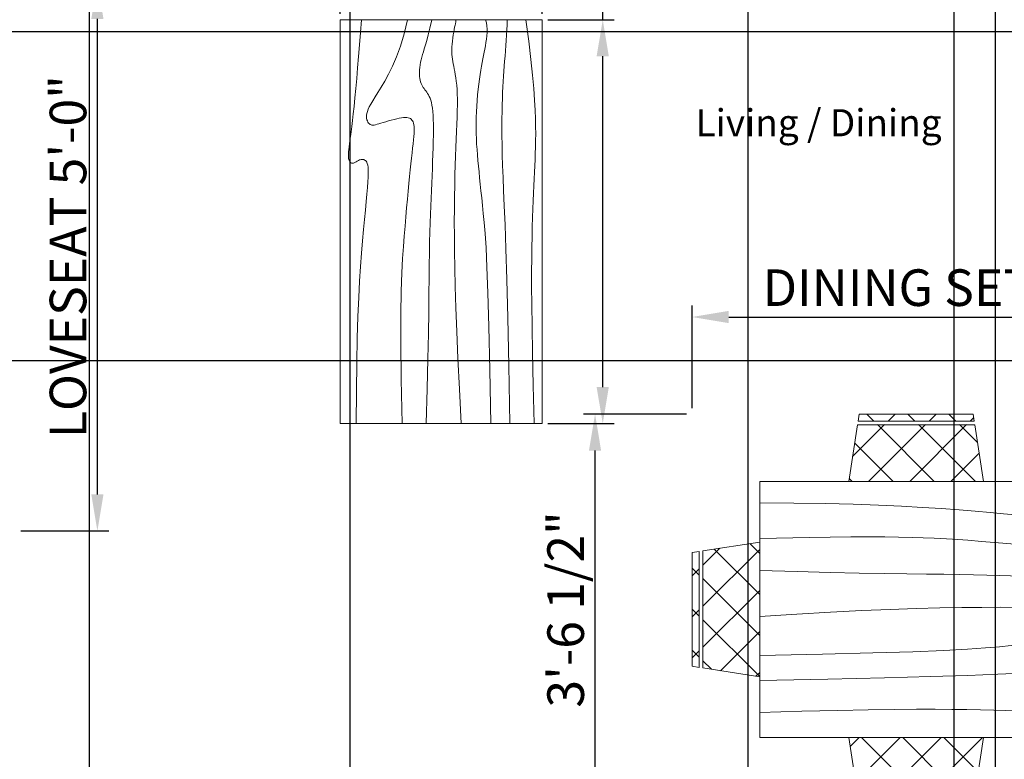
# Model space of a CAD drawing. Units: inches. Extents: x 1872 to 2380, y 714 to 1327.
# Tile 5 of 9: x 1994 to 2101, y 974 to 1055. Entities that reach past the tile are written whole.
import ezdxf

# ---------------------------------------------------------------- set-up
doc = ezdxf.new("R2010")
doc.units = ezdxf.units.IN
for name, color, linetype, lineweight in [('A-ANNO-DIMS', 2, 'Continuous', 18), ('A-AREA-IDEN', 7, 'Continuous', 18), ('A-FURN', 8, 'Continuous', 18)]:
    doc.layers.add(name, color=color, linetype=linetype, lineweight=lineweight)
doc.layers.add('A-FURN-PATT', color=254, linetype='Continuous', lineweight=13, true_color=0xf8ceb3)
doc.styles.get("Standard").update_dxf_attribs({"font": 'arial.ttf'})
doc.dimstyles.new('ISO-25', dxfattribs={"dimtxt": 4, "dimasz": 4, "dimexe": 1.25, "dimexo": 0.625, "dimtad": 1, "dimdec": 0, "dimlunit": 3, "dimtxsty": 'Standard', "dimcen": 2.5, "dimadec": 0, "dimazin": 0, "dimtfac": 1, "dimtdec": 0, "dimtmove": 0, "dimatfit": 3, "dimfxl": 1, "dimarcsym": 0})

# ---------------------------------------------------------------- blocks, each defined once
blk = doc.blocks.new('Table - Rectangular Woodgrain 60 x 30 in.')
for p, q in [((0, 0), (0, -30)), ((60, 0), (0, 0)), ((60, -30), (60, 0)), ((0, -30), (60, -30))]:
    blk.add_line(p, q)
for points in [[(0, -2.4), (4.8155, -2.418), (9.0302, -2.4688), (12.709, -2.5477), (15.9167, -2.65), (18.7181, -2.7711), (21.1781, -2.9063), (23.3616, -3.0508), (25.3333, -3.2), (27.1477, -3.3495), (28.8172, -3.4958), (30.3437, -3.636), (31.7291, -3.7667), (32.9756, -3.8849), (34.0849, -3.9875), (35.059, -4.0714), (35.9, -4.1334), (36.6114, -4.1711), (37.2041, -4.1854), (37.6906, -4.1779), (38.0833, -4.15), (38.3948, -4.1034), (38.6375, -4.0396), (38.8239, -3.9602), (38.9666, -3.8667), (39.0764, -3.7608), (39.1573, -3.6448), (39.2116, -3.521), (39.2416, -3.3917), (39.2498, -3.2593), (39.2385, -3.1261), (39.21, -2.9944), (39.1666, -2.8667), (39.111, -2.7447), (39.0468, -2.6281), (38.978, -2.5163), (38.9083, -2.4083), (38.8418, -2.3035), (38.7823, -2.201), (38.7337, -2.1001), (38.7, -2), (38.6844, -1.9003), (38.6875, -1.8021), (38.7094, -1.707), (38.75, -1.6167), (38.8094, -1.5326), (38.8875, -1.4563), (38.9844, -1.3893), (39.1, -1.3333), (39.2351, -1.2896), (39.3937, -1.2583), (39.5804, -1.2396), (39.8, -1.2333), (40.057, -1.2396), (40.3562, -1.2583), (40.7023, -1.2896), (41.1, -1.3333), (41.5547, -1.3895), (42.0755, -1.4573), (42.6721, -1.5361), (43.3542, -1.625), (44.1316, -1.7233), (45.014, -1.8302), (46.0114, -1.9449), (47.1333, -2.0667), (48.3862, -2.1947), (49.7625, -2.3281), (51.2513, -2.4663), (52.8416, -2.6083), (54.5226, -2.7535), (56.2833, -2.9011), (58.1127, -3.0501), (60, -3.2)], [(0, -9.2), (6.5759, -9.0858), (11.9385, -9.0365), (16.2527, -9.0418), (19.6833, -9.0917), (22.3952, -9.1759), (24.5531, -9.2844), (26.322, -9.4069), (27.8666, -9.5333), (29.3241, -9.6553), (30.7203, -9.7719), (32.0532, -9.8837), (33.3208, -9.9917), (34.5213, -10.0965), (35.6526, -10.199), (36.7128, -10.2999), (37.7, -10.4), (38.6129, -10.4996), (39.4531, -10.5969), (40.223, -10.6895), (40.925, -10.775), (41.5613, -10.8512), (42.1344, -10.9156), (42.6465, -10.966), (43.1, -11), (43.4976, -11.0158), (43.8437, -11.0136), (44.143, -10.9942), (44.4, -10.9583), (44.6195, -10.9069), (44.8062, -10.8406), (44.9648, -10.7603), (45.1, -10.6667), (45.2155, -10.5598), (45.3114, -10.4365), (45.3871, -10.2929), (45.4416, -10.125), (45.4743, -9.929), (45.4844, -9.7011), (45.4709, -9.4371), (45.4333, -9.1333), (45.3716, -8.7883), (45.2896, -8.4104), (45.1919, -8.0107), (45.0833, -7.6), (44.9685, -7.1893), (44.8521, -6.7896), (44.7388, -6.4117), (44.6333, -6.0667), (44.54, -5.7628), (44.4614, -5.4979), (44.4001, -5.2675), (44.3583, -5.0667), (44.3384, -4.8909), (44.3427, -4.7354), (44.3736, -4.5956), (44.4333, -4.4667), (44.5236, -4.3453), (44.6427, -4.2333), (44.7884, -4.1339), (44.9583, -4.05), (45.1501, -3.9849), (45.3614, -3.9417), (45.59, -3.9234), (45.8333, -3.9333), (46.0915, -3.9749), (46.3734, -4.0531), (46.6906, -4.1736), (47.0542, -4.3417), (47.4756, -4.5629), (47.9661, -4.8427), (48.5372, -5.1866), (49.2, -5.6), (49.9676, -6.0844), (50.8594, -6.625), (51.8965, -7.2031), (53.1, -7.8), (54.491, -8.3969), (56.0906, -8.975), (57.9199, -9.5156), (60, -10)], [(0, -12.8), (5.1847, -12.9322), (9.6213, -13.0323), (13.3963, -13.1059), (16.5958, -13.1583), (19.3063, -13.1952), (21.614, -13.2219), (23.6054, -13.2439), (25.3666, -13.2667), (26.9728, -13.2947), (28.4531, -13.3281), (29.8256, -13.3663), (31.1083, -13.4083), (32.3191, -13.4535), (33.476, -13.501), (34.597, -13.5501), (35.7, -13.6), (36.7984, -13.6497), (37.8875, -13.6979), (38.9578, -13.743), (40, -13.7833), (41.0047, -13.8174), (41.9625, -13.8438), (42.864, -13.8607), (43.7, -13.8667), (44.4631, -13.8604), (45.1552, -13.8417), (45.7801, -13.8104), (46.3416, -13.7667), (46.8439, -13.7104), (47.2906, -13.6417), (47.6858, -13.5604), (48.0333, -13.4667), (48.3375, -13.3608), (48.6042, -13.2448), (48.8396, -13.121), (49.05, -12.9917), (49.2417, -12.8593), (49.4208, -12.7261), (49.5937, -12.5944), (49.7667, -12.4667), (49.9452, -12.3451), (50.1323, -12.2313), (50.3303, -12.1268), (50.5416, -12.0333), (50.7686, -11.9524), (51.0135, -11.8854), (51.2788, -11.8341), (51.5666, -11.8), (51.8785, -11.7843), (52.2116, -11.7865), (52.562, -11.8059), (52.926, -11.8417), (53.2998, -11.8931), (53.6795, -11.9594), (54.0614, -12.0397), (54.4416, -12.1333), (54.8223, -12.2401), (55.2293, -12.3625), (55.6942, -12.5037), (56.2489, -12.6667), (56.9251, -12.8547), (57.7545, -13.0708), (58.7689, -13.3182), (60, -13.6)], [(0, -18), (5.124, -17.7273), (9.6609, -17.5057), (13.6705, -17.3303), (17.2125, -17.1958), (20.3467, -17.0973), (23.1328, -17.0297), (25.6307, -16.9878), (27.9, -16.9667), (29.9928, -16.9617), (31.9302, -16.9703), (33.7254, -16.9907), (35.3917, -17.0208), (36.9423, -17.0588), (38.3906, -17.1026), (39.7499, -17.1503), (41.0333, -17.2), (42.2519, -17.2496), (43.4073, -17.2969), (44.4986, -17.3395), (45.525, -17.375), (46.4858, -17.4012), (47.3802, -17.4156), (48.2074, -17.416), (48.9667, -17.4), (49.6583, -17.3662), (50.2872, -17.3167), (50.8595, -17.2547), (51.3812, -17.1833), (51.8584, -17.1057), (52.2971, -17.025), (52.7034, -16.9443), (53.0833, -16.8667), (53.443, -16.7951), (53.789, -16.7313), (54.128, -16.6768), (54.4666, -16.6334), (54.8115, -16.6024), (55.1693, -16.5854), (55.5465, -16.5841), (55.95, -16.6), (56.3828, -16.6337), (56.8346, -16.6823), (57.2915, -16.7418), (57.7396, -16.8084), (58.165, -16.878), (58.5539, -16.9469), (58.8924, -17.0111), (59.1666, -17.0667), (59.3679, -17.1107), (59.5078, -17.1438), (59.6032, -17.1675), (59.6708, -17.1833), (59.7275, -17.193), (59.7901, -17.1979), (59.8753, -17.1998), (60, -17.2)], [(0, -22.4), (8.0098, -22.2501), (14.4094, -22.1011), (19.4168, -21.9535), (23.25, -21.8083), (26.1269, -21.6663), (28.2656, -21.5281), (29.884, -21.3947), (31.2, -21.2667), (32.3967, -21.1448), (33.5172, -21.0292), (34.5697, -20.9198), (35.5625, -20.8167), (36.5037, -20.7198), (37.4015, -20.6292), (38.2642, -20.5448), (39.1, -20.4667), (39.9164, -20.3951), (40.7187, -20.3313), (41.5117, -20.2768), (42.3, -20.2333), (43.0883, -20.2024), (43.8812, -20.1854), (44.6836, -20.1841), (45.5, -20.2), (46.3328, -20.234), (47.1747, -20.2844), (48.0163, -20.3488), (48.8479, -20.425), (49.66, -20.5106), (50.4429, -20.6031), (51.1872, -20.7004), (51.8833, -20.8), (52.5246, -20.8999), (53.1166, -20.9995), (53.6681, -21.0983), (54.1875, -21.1958), (54.6834, -21.2919), (55.1646, -21.3859), (55.6394, -21.4777), (56.1167, -21.5667), (56.6028, -21.6515), (57.0961, -21.7266), (57.5929, -21.7852), (58.0896, -21.8208), (58.5823, -21.8268), (59.0674, -21.7964), (59.5412, -21.723), (60, -21.6)], [(0, -25.2), (8.6355, -25.0504), (15.7026, -24.9031), (21.4049, -24.7606), (25.9458, -24.625), (29.529, -24.4988), (32.3578, -24.3844), (34.6359, -24.284), (36.5667, -24.2), (38.3213, -24.1341), (39.9417, -24.0854), (41.437, -24.0523), (42.8167, -24.0333), (44.0901, -24.0268), (45.2667, -24.0313), (46.3557, -24.0451), (47.3667, -24.0667), (48.309, -24.0947), (49.1928, -24.1287), (50.0284, -24.168), (50.826, -24.2125), (51.5959, -24.2617), (52.3483, -24.3151), (53.0935, -24.3725), (53.8417, -24.4334), (54.6009, -24.497), (55.3699, -24.561), (56.1454, -24.6226), (56.9239, -24.6792), (57.7021, -24.7279), (58.4764, -24.7662), (59.2435, -24.7911), (60, -24.8)], [(0, -28.8), (5.6867, -28.6681), (10.45, -28.5698), (14.407, -28.5012), (17.675, -28.4584), (20.3711, -28.4374), (22.6125, -28.4344), (24.5164, -28.4455), (26.2, -28.4667), (27.762, -28.4947), (29.2276, -28.5281), (30.6033, -28.5663), (31.8958, -28.6084), (33.1118, -28.6535), (34.2578, -28.7011), (35.3405, -28.7501), (36.3666, -28.8), (37.3443, -28.8497), (38.288, -28.8974), (39.2137, -28.9412), (40.1375, -28.9792), (41.0753, -29.0093), (42.0432, -29.0297), (43.0572, -29.0384), (44.1333, -29.0333), (45.2936, -29.0114), (46.5843, -28.9641), (48.0579, -28.8816), (49.7666, -28.7542), (51.7629, -28.5721), (54.0989, -28.3255), (56.8272, -28.0048), (60, -27.6)]]:
    blk.add_lwpolyline(points)
blk = doc.blocks.new('Dining Set - 36 x 72 in.')
for p, q in [((-22, 27.5), (-22.1562, 26.50042)), ((-5.8416, 26.5), (-22.1534, 26.5)), ((-22, 27.5), (-6, 27.5)), ((-5.8437, 26.49966), (-6, 27.5)), ((6, 27.5), (5.8438, 26.50042)), ((22.1584, 26.5), (5.8466, 26.5)), ((6, 27.5), (22, 27.5)), ((22.1563, 26.49966), (22, 27.5)), ((-22.2343, 26.00059), (-23.4847, 17.99762)), ((-22.2304, 26), (-5.7608, 26)), ((-4.5152, 17.99762), (-5.7655, 25.99926)), ((5.7657, 26.00059), (4.5153, 17.99762)), ((5.7696, 26), (22.2392, 26)), ((23.4848, 17.99762), (22.2345, 25.99926)), ((36, 18), (-36, 18)), ((-36, 18), (-36, -18)), ((36, -18), (36, 18)), ((-44.0006, 8.23428), (-35.9976, 9.48474)), ((44.0006, 8.23428), (35.9976, 9.48474)), ((-45.5, 8), (-44.5004, 8.15617)), ((-45.5, 8), (-45.5, -8)), ((-44.5, -8.15843), (-44.5, 8.15338)), ((-44, 8.23041), (-44, -8.23915)), ((44, 8.23041), (44, -8.23915)), ((44.5, -8.15843), (44.5, 8.15338)), ((45.5, 8), (44.5005, 8.15617)), ((45.5, 8), (45.5, -8)), ((-44.4997, -8.15631), (-45.5, -8)), ((-35.9976, -9.48476), (-43.9993, -8.2345)), ((35.9976, -9.48476), (43.9993, -8.2345)), ((44.4997, -8.15631), (45.5, -8)), ((-36, -18), (36, -18)), ((-22.2343, -26.0006), (-23.4847, -17.99762)), ((-4.5152, -17.99762), (-5.7655, -25.99928)), ((5.7657, -26.0006), (4.5153, -17.99762)), ((23.4848, -17.99762), (22.2345, -25.99928)), ((-22.2304, -26), (-5.7608, -26)), ((5.7696, -26), (22.2392, -26)), ((-22, -27.5), (-22.1562, -26.50044)), ((-5.8416, -26.5), (-22.1534, -26.5)), ((-22, -27.5), (-6, -27.5)), ((-5.8437, -26.49967), (-6, -27.5)), ((6, -27.5), (5.8438, -26.50044)), ((22.1584, -26.5), (5.8466, -26.5)), ((6, -27.5), (22, -27.5)), ((22.1563, -26.49967), (22, -27.5))]:
    blk.add_line(p, q)
for points in [[(-36, 15), (-31.1772, 14.97754), (-26.8079, 14.91406), (-22.8538, 14.81543), (-19.276, 14.6875), (-16.0362, 14.53613), (-13.0957, 14.36718), (-10.4159, 14.18652), (-7.9583, 14), (-5.6904, 13.81315), (-3.6035, 13.63021), (-1.6954, 13.45508), (0.0365, 13.29166), (1.5945, 13.14388), (2.9811, 13.01562), (4.1988, 12.9108), (5.25, 12.83333), (6.1393, 12.78613), (6.8802, 12.76823), (7.4883, 12.77767), (7.9792, 12.8125), (8.3685, 12.87077), (8.6719, 12.95052), (8.9049, 13.0498), (9.0833, 13.16666), (9.2205, 13.29899), (9.3216, 13.44401), (9.3895, 13.59879), (9.4271, 13.76041), (9.4373, 13.92594), (9.4232, 14.09245), (9.3875, 14.257), (9.3333, 14.41666), (9.2638, 14.56917), (9.1836, 14.71484), (9.0975, 14.85465), (9.0104, 14.98958), (8.9272, 15.1206), (8.8529, 15.2487), (8.7922, 15.37483), (8.75, 15.5), (8.7305, 15.62467), (8.7344, 15.74739), (8.7617, 15.86621), (8.8125, 15.97916), (8.8867, 16.08431), (8.9844, 16.17968), (9.1055, 16.26334), (9.25, 16.33333), (9.4189, 16.38802), (9.6172, 16.42708), (9.8506, 16.45052), (10.125, 16.45833), (10.4463, 16.45052), (10.8203, 16.42708), (11.2529, 16.38802), (11.75, 16.33333), (12.3184, 16.26318), (12.9694, 16.17838), (13.7151, 16.07991), (14.5677, 15.96875), (15.5395, 15.84586), (16.6426, 15.71224), (17.8893, 15.56884), (19.2917, 15.41666), (20.859, 15.25667), (22.5879, 15.08984), (24.4721, 14.91715), (26.5052, 14.73958), (28.6809, 14.5581), (30.9929, 14.3737), (33.4347, 14.18733), (36, 14)], [(-36, 10), (-28.9766, 10.14274), (-23.1725, 10.20442), (-18.4241, 10.19775), (-14.5677, 10.13541), (-11.4399, 10.03011), (-8.877, 9.89453), (-6.7154, 9.74137), (-4.7917, 9.58333), (-2.9698, 9.43082), (-1.2246, 9.28515), (0.4415, 9.14534), (2.026, 9.01041), (3.5266, 8.87939), (4.9408, 8.7513), (6.266, 8.62516), (7.5, 8.5), (8.6411, 8.37549), (9.6914, 8.2539), (10.6538, 8.13818), (11.5312, 8.03125), (12.3267, 7.93603), (13.043, 7.85547), (13.6831, 7.79248), (14.25, 7.75), (14.7471, 7.7303), (15.1797, 7.73307), (15.5537, 7.75732), (15.875, 7.80208), (16.1494, 7.86637), (16.3828, 7.94922), (16.5811, 8.04964), (16.75, 8.16666), (16.8944, 8.29915), (17.0143, 8.44531), (17.1089, 8.60319), (17.1771, 8.77083), (17.218, 8.94629), (17.2305, 9.1276), (17.2137, 9.31282), (17.1667, 9.5), (17.0895, 9.6875), (16.987, 9.875), (16.8649, 10.0625), (16.7292, 10.25), (16.5856, 10.4375), (16.4401, 10.625), (16.2985, 10.8125), (16.1667, 11), (16.05, 11.18733), (15.9518, 11.3737), (15.8752, 11.5581), (15.8229, 11.73958), (15.798, 11.91715), (15.8034, 12.08984), (15.842, 12.25667), (15.9167, 12.41666), (16.0295, 12.56836), (16.1784, 12.70833), (16.3605, 12.83268), (16.5729, 12.9375), (16.8127, 13.01888), (17.0768, 13.07291), (17.3625, 13.0957), (17.6667, 13.08333), (17.9894, 13.03312), (18.3418, 12.94726), (18.7382, 12.82918), (19.1927, 12.68229), (19.7195, 12.51001), (20.3327, 12.31575), (21.0465, 12.10294), (21.875, 11.875), (22.8357, 11.63354), (23.959, 11.37304), (25.2786, 11.08618), (26.8282, 10.76562), (28.6414, 10.40405), (30.752, 9.99414), (33.1936, 9.52856), (36, 9)], [(-36, 5.5), (-30.7157, 5.3348), (-26.069, 5.20963), (-21.9946, 5.11767), (-18.4271, 5.05208), (-15.3009, 5.00602), (-12.5508, 4.97265), (-10.1112, 4.94515), (-7.9167, 4.91666), (-5.909, 4.88167), (-4.0586, 4.83984), (-2.3429, 4.79215), (-0.7396, 4.73958), (0.7739, 4.6831), (2.22, 4.6237), (3.6213, 4.56233), (5, 4.5), (6.373, 4.43782), (7.7344, 4.3776), (9.0723, 4.32129), (10.375, 4.27083), (11.6309, 4.22819), (12.8281, 4.19531), (13.9551, 4.17415), (15, 4.16666), (15.954, 4.17448), (16.819, 4.19791), (17.6001, 4.23698), (18.3021, 4.29166), (18.9299, 4.36198), (19.4883, 4.44791), (19.9823, 4.54948), (20.4167, 4.66666), (20.7969, 4.79899), (21.1302, 4.94401), (21.4245, 5.09879), (21.6875, 5.26041), (21.9271, 5.42594), (22.1511, 5.59245), (22.3672, 5.757), (22.5834, 5.91666), (22.8065, 6.06868), (23.0404, 6.21093), (23.2879, 6.34147), (23.5521, 6.45833), (23.8358, 6.55957), (24.142, 6.64323), (24.4735, 6.70735), (24.8334, 6.75), (25.2235, 6.76969), (25.642, 6.76692), (26.0858, 6.74267), (26.5521, 6.69791), (27.0379, 6.63362), (27.5404, 6.55078), (28.0565, 6.45036), (28.5834, 6.33333), (29.1242, 6.19987), (29.7071, 6.04687), (30.3661, 5.87044), (31.1354, 5.66666), (32.0493, 5.43164), (33.142, 5.16146), (34.4475, 4.85221), (36, 4.5)], [(-36, -1), (-30.7915, -0.6591), (-26.0195, -0.38216), (-21.6519, -0.16284), (-17.6563, 0.00521), (-14.0005, 0.12833), (-10.6523, 0.21289), (-7.5796, 0.26522), (-4.75, 0.29166), (-2.134, 0.29793), (0.2878, 0.28711), (2.5317, 0.26163), (4.6146, 0.22396), (6.5529, 0.17651), (8.3633, 0.12174), (10.0623, 0.06209), (11.6667, 0), (13.1899, -0.06201), (14.6341, -0.1211), (15.9982, -0.17432), (17.2813, -0.21875), (18.4823, -0.25147), (19.6003, -0.26953), (20.6343, -0.27002), (21.5834, -0.25), (22.4481, -0.20768), (23.2357, -0.14584), (23.9549, -0.06836), (24.6146, 0.02083), (25.2235, 0.11784), (25.7904, 0.21875), (26.3241, 0.31966), (26.8334, 0.41666), (27.3265, 0.50618), (27.8099, 0.58593), (28.2894, 0.65397), (28.7709, 0.70833), (29.2601, 0.74707), (29.763, 0.76823), (30.2855, 0.76985), (30.8334, 0.75), (31.4088, 0.70784), (31.9994, 0.64713), (32.589, 0.57275), (33.1615, 0.48958), (33.7008, 0.4025), (34.1908, 0.3164), (34.6153, 0.23616), (34.9584, 0.16666), (35.2099, 0.11165), (35.3848, 0.07031), (35.504, 0.04069), (35.5886, 0.02083), (35.6594, 0.00879), (35.7377, 0.0026), (35.8442, 0.00032), (36, 0)], [(-36, -6.5), (-27.1843, -6.31267), (-20.084, -6.1263), (-14.469, -5.9419), (-10.1094, -5.76042), (-6.7752, -5.58285), (-4.2363, -5.41016), (-2.2629, -5.24333), (-0.625, -5.08334), (0.8708, -4.93099), (2.2715, -4.78646), (3.5872, -4.64974), (4.8281, -4.52084), (6.0046, -4.39974), (7.127, -4.28646), (8.2053, -4.18099), (9.25, -4.08334), (10.2705, -3.99382), (11.2734, -3.91407), (12.2647, -3.84603), (13.25, -3.79167), (14.2354, -3.75293), (15.2266, -3.73177), (16.2295, -3.73015), (17.25, -3.75), (18.2912, -3.79248), (19.3451, -3.85547), (20.4009, -3.93604), (21.4479, -4.03125), (22.4754, -4.13819), (23.4727, -4.25391), (24.4289, -4.37549), (25.3334, -4.5), (26.1785, -4.62492), (26.9694, -4.74935), (27.7145, -4.87281), (28.4219, -4.99479), (29.1, -5.11483), (29.7572, -5.23242), (30.4016, -5.34709), (31.0417, -5.45834), (31.6837, -5.56437), (32.3262, -5.65821), (32.9658, -5.73153), (33.599, -5.77604), (34.2224, -5.78345), (34.8327, -5.74545), (35.4264, -5.65373), (36, -5.5)], [(-36, -10), (-26.4022, -9.81299), (-18.4675, -9.62891), (-11.9839, -9.45069), (-6.7396, -9.28125), (-2.5226, -9.12354), (0.8789, -8.98047), (3.6769, -8.85498), (6.0833, -8.75), (8.2767, -8.66765), (10.3021, -8.60677), (12.1712, -8.56543), (13.8958, -8.54167), (15.4876, -8.53353), (16.9583, -8.53907), (18.3197, -8.55632), (19.5834, -8.58334), (20.7616, -8.61841), (21.8685, -8.66081), (22.9188, -8.71004), (23.9271, -8.76563), (24.9081, -8.82707), (25.8763, -8.89388), (26.8465, -8.96558), (27.8334, -9.04167), (28.8474, -9.12118), (29.8828, -9.20117), (30.93, -9.27824), (31.9792, -9.34896), (33.0205, -9.40991), (34.0443, -9.45768), (35.0407, -9.48885), (36, -9.5)], [(-36, -14.5), (-30.0881, -14.33513), (-25.0332, -14.21224), (-20.7312, -14.12647), (-17.0781, -14.07292), (-13.97, -14.04671), (-11.3027, -14.04297), (-8.9724, -14.05681), (-6.875, -14.08334), (-4.9224, -14.11833), (-3.0905, -14.16016), (-1.3709, -14.20785), (0.2448, -14.26042), (1.7647, -14.3169), (3.1973, -14.3763), (4.5507, -14.43767), (5.8333, -14.5), (7.0554, -14.5621), (8.235, -14.62175), (9.3922, -14.67652), (10.5469, -14.72396), (11.7192, -14.76164), (12.929, -14.78711), (14.1965, -14.79794), (15.5417, -14.79167), (16.9933, -14.76424), (18.6152, -14.70508), (20.4804, -14.60197), (22.6615, -14.44271), (25.2312, -14.21509), (28.2624, -13.9069), (31.8277, -13.50594), (36, -13)]]:
    blk.add_lwpolyline(points)
blk = doc.blocks.new('*D40')
at = {"layer": 'A-ANNO-DIMS', "color": 0, "lineweight": -2, "transparency": 16777216}
for p, q in [((1993.9, 1059.04), (2003.52, 1059.04)), ((2002.27, 1003.04), (2002.27, 1055.04)), ((1993.9, 999.04), (2003.52, 999.04))]:
    blk.add_line(p, q, dxfattribs=at)
at = {"layer": 'A-ANNO-DIMS', "color": 0, "transparency": 16777216}
for points in [[(2001.61, 1055.04), (2002.94, 1055.04), (2002.27, 1059.04)], [(2001.61, 1003.04), (2002.94, 1003.04), (2002.27, 999.04)]]:
    blk.add_solid(points, dxfattribs=at)
at = {"layer": 'Defpoints', "color": 0, "transparency": 16777216}
for p in [(1993.27, 1059.04), (2002.27, 1059.04), (1993.27, 999.04)]:
    blk.add_point(p, dxfattribs=at)
at = {"layer": 'A-ANNO-DIMS', "color": 0, "transparency": 16777216, "insert": (1999.58, 1029.04), "char_height": 4, "attachment_point": 5, "rotation": 90}
blk.add_mtext('LOVESEAT 5\'-0"', dxfattribs=at)
blk = doc.blocks.new('*D44')
at = {"layer": 'A-ANNO-DIMS', "color": 0, "lineweight": -2, "transparency": 16777216}
for p, q in [((2057.51, 1054.95), (2057.51, 1114.26)), ((2051.51, 1054.95), (2058.76, 1054.95)), ((2057.51, 1014.78), (2057.51, 1050.95)), ((2051.51, 1010.78), (2058.76, 1010.78))]:
    blk.add_line(p, q, dxfattribs=at)
at = {"layer": 'A-ANNO-DIMS', "color": 0, "transparency": 16777216}
for points in [[(2056.84, 1050.95), (2058.17, 1050.95), (2057.51, 1054.95)], [(2056.84, 1014.78), (2058.17, 1014.78), (2057.51, 1010.78)]]:
    blk.add_solid(points, dxfattribs=at)
at = {"layer": 'Defpoints', "color": 0, "transparency": 16777216}
for p in [(2050.88, 1054.95), (2057.51, 1054.95), (2050.88, 1010.78)]:
    blk.add_point(p, dxfattribs=at)
at = {"layer": 'A-ANNO-DIMS', "color": 0, "transparency": 16777216, "insert": (2054.81, 1086.61), "char_height": 4, "attachment_point": 5, "rotation": 90}
blk.add_mtext('COFFEE TABLE 3\'-8"', dxfattribs=at)
blk = doc.blocks.new('*D45')
at = {"layer": 'A-ANNO-DIMS', "color": 0, "lineweight": -2, "transparency": 16777216}
for p, q in [((2028.8, 1055.58), (2028.8, 1062.83)), ((2050.88, 1055.58), (2050.88, 1062.83)), ((2046.88, 1061.58), (2032.8, 1061.58))]:
    blk.add_line(p, q, dxfattribs=at)
at = {"layer": 'A-ANNO-DIMS', "color": 0, "transparency": 16777216}
for points in [[(2032.8, 1062.25), (2032.8, 1060.91), (2028.8, 1061.58)], [(2046.88, 1062.25), (2046.88, 1060.91), (2050.88, 1061.58)]]:
    blk.add_solid(points, dxfattribs=at)
at = {"layer": 'Defpoints', "color": 0, "transparency": 16777216}
for p in [(2028.8, 1061.58), (2028.8, 1054.95), (2050.88, 1054.95)]:
    blk.add_point(p, dxfattribs=at)
at = {"layer": 'A-ANNO-DIMS', "color": 0, "transparency": 16777216, "insert": (2039.84, 1064.25), "char_height": 4, "attachment_point": 5}
blk.add_mtext('1\'-10"', dxfattribs=at)
blk = doc.blocks.new('*D46')
at = {"layer": 'A-ANNO-DIMS', "color": 0, "lineweight": -2, "transparency": 16777216}
for p, q in [((2067.28, 1012.46), (2067.28, 1023.69)), ((2137.99, 1012.46), (2137.99, 1023.69)), ((2071.28, 1022.44), (2133.99, 1022.44))]:
    blk.add_line(p, q, dxfattribs=at)
at = {"layer": 'A-ANNO-DIMS', "color": 0, "transparency": 16777216}
for points in [[(2071.28, 1023.11), (2071.28, 1021.77), (2067.28, 1022.44)], [(2133.99, 1023.11), (2133.99, 1021.77), (2137.99, 1022.44)]]:
    blk.add_solid(points, dxfattribs=at)
at = {"layer": 'Defpoints', "color": 0, "transparency": 16777216}
for p in [(2137.99, 1022.44), (2067.28, 1011.83), (2137.99, 1011.83)]:
    blk.add_point(p, dxfattribs=at)
at = {"layer": 'A-ANNO-DIMS', "color": 0, "transparency": 16777216, "insert": (2102.64, 1025.13), "char_height": 4, "attachment_point": 5}
blk.add_mtext('DINING SET 5\'-10 1/2"', dxfattribs=at)
blk = doc.blocks.new('*D47')
at = {"layer": 'A-ANNO-DIMS', "color": 0, "lineweight": -2, "transparency": 16777216}
for p, q in [((2066.65, 1011.83), (2055.42, 1011.83)), ((2056.67, 973.09), (2056.67, 1007.83)), ((2066.65, 969.09), (2055.42, 969.09))]:
    blk.add_line(p, q, dxfattribs=at)
at = {"layer": 'A-ANNO-DIMS', "color": 0, "transparency": 16777216}
for points in [[(2056, 1007.83), (2057.33, 1007.83), (2056.67, 1011.83)], [(2056, 973.09), (2057.33, 973.09), (2056.67, 969.09)]]:
    blk.add_solid(points, dxfattribs=at)
at = {"layer": 'Defpoints', "color": 0, "transparency": 16777216}
for p in [(2056.67, 1011.83), (2067.28, 1011.83), (2067.28, 969.09)]:
    blk.add_point(p, dxfattribs=at)
at = {"layer": 'A-ANNO-DIMS', "color": 0, "transparency": 16777216, "insert": (2053.97, 990.46), "char_height": 4, "attachment_point": 5, "rotation": 90}
blk.add_mtext('3\'-6 1/2"', dxfattribs=at)
blk = doc.blocks.new('*D67')
at = {"layer": 'A-ANNO-DIMS', "color": 0, "lineweight": -2, "transparency": 16777216}
for p, q in [((1943.77, 1112.77), (1905.35, 1112.77)), ((1906.6, 956.99), (1906.6, 1108.77)), ((2000.77, 952.99), (1905.35, 952.99))]:
    blk.add_line(p, q, dxfattribs=at)
at = {"layer": 'A-ANNO-DIMS', "color": 0, "transparency": 16777216}
for points in [[(1905.93, 1108.77), (1907.27, 1108.77), (1906.6, 1112.77)], [(1905.93, 956.99), (1907.27, 956.99), (1906.6, 952.99)]]:
    blk.add_solid(points, dxfattribs=at)
at = {"layer": 'Defpoints', "color": 0, "transparency": 16777216}
for p in [(1906.6, 1112.77), (1944.4, 1112.77), (2001.4, 952.99)]:
    blk.add_point(p, dxfattribs=at)
at = {"layer": 'A-ANNO-DIMS', "color": 0, "transparency": 16777216, "insert": (1903.93, 1032.88), "char_height": 4, "attachment_point": 5, "rotation": 90}
blk.add_mtext('13\'-4"', dxfattribs=at)
blk = doc.blocks.new('*D73')
at = {"layer": 'A-ANNO-DIMS', "color": 0, "lineweight": -2, "transparency": 16777216}
for p, q in [((2197.27, 1053.64), (1905.35, 1053.64)), ((1906.6, 1021.64), (1906.6, 1049.64)), ((2197.27, 1017.64), (1905.35, 1017.64))]:
    blk.add_line(p, q, dxfattribs=at)
at = {"layer": 'A-ANNO-DIMS', "color": 0, "transparency": 16777216}
for points in [[(1905.93, 1049.64), (1907.27, 1049.64), (1906.6, 1053.64)], [(1905.93, 1021.64), (1907.27, 1021.64), (1906.6, 1017.64)]]:
    blk.add_solid(points, dxfattribs=at)
at = {"layer": 'Defpoints', "color": 0, "transparency": 16777216}
for p in [(1906.6, 1053.64), (2197.9, 1053.64), (2197.9, 1017.64)]:
    blk.add_point(p, dxfattribs=at)
at = {"layer": 'A-ANNO-DIMS', "color": 0, "transparency": 16777216, "insert": (1903.93, 1035.64), "char_height": 4, "attachment_point": 5, "rotation": 90}
blk.add_mtext('3\'-0"', dxfattribs=at)
blk = doc.blocks.new('*D76')
at = {"layer": 'A-ANNO-DIMS', "color": 0, "lineweight": -2, "transparency": 16777216}
for p, q in [((2001.4, 953.62), (2001.4, 1319.69)), ((2029.9, 953.62), (2029.9, 1319.69)), ((2005.4, 1318.44), (2025.9, 1318.44))]:
    blk.add_line(p, q, dxfattribs=at)
at = {"layer": 'A-ANNO-DIMS', "color": 0, "transparency": 16777216}
for points in [[(2005.4, 1319.11), (2005.4, 1317.78), (2001.4, 1318.44)], [(2025.9, 1319.11), (2025.9, 1317.78), (2029.9, 1318.44)]]:
    blk.add_solid(points, dxfattribs=at)
at = {"layer": 'Defpoints', "color": 0, "transparency": 16777216}
for p in [(2029.9, 1318.44), (2001.4, 952.99), (2029.9, 952.99)]:
    blk.add_point(p, dxfattribs=at)
at = {"layer": 'A-ANNO-DIMS', "color": 0, "transparency": 16777216, "insert": (2015.65, 1321.14), "char_height": 4, "attachment_point": 5}
blk.add_mtext('2\'-4 1/2"', dxfattribs=at)
blk = doc.blocks.new('*D77')
at = {"layer": 'A-ANNO-DIMS', "color": 0, "lineweight": -2, "transparency": 16777216}
for p, q in [((2029.9, 953.62), (2029.9, 1319.69)), ((2073.4, 953.62), (2073.4, 1319.69)), ((2033.9, 1318.44), (2069.4, 1318.44))]:
    blk.add_line(p, q, dxfattribs=at)
at = {"layer": 'A-ANNO-DIMS', "color": 0, "transparency": 16777216}
for points in [[(2033.9, 1319.11), (2033.9, 1317.78), (2029.9, 1318.44)], [(2069.4, 1319.11), (2069.4, 1317.78), (2073.4, 1318.44)]]:
    blk.add_solid(points, dxfattribs=at)
at = {"layer": 'Defpoints', "color": 0, "transparency": 16777216}
for p in [(2073.4, 1318.44), (2029.9, 952.99), (2073.4, 952.99)]:
    blk.add_point(p, dxfattribs=at)
at = {"layer": 'A-ANNO-DIMS', "color": 0, "transparency": 16777216, "insert": (2051.65, 1321.14), "char_height": 4, "attachment_point": 5}
blk.add_mtext('3\'-7 1/2"', dxfattribs=at)
blk = doc.blocks.new('*D80')
at = {"layer": 'A-ANNO-DIMS', "color": 0, "lineweight": -2, "transparency": 16777216}
for p, q in [((2095.9, 1112.15), (2095.9, 716.39)), ((2100.4, 1112.15), (2100.4, 716.39)), ((2091.9, 717.64), (2087.9, 717.64)), ((2095.9, 717.64), (2100.4, 717.64)), ((2104.4, 717.64), (2129.6, 717.64))]:
    blk.add_line(p, q, dxfattribs=at)
at = {"layer": 'A-ANNO-DIMS', "color": 0, "transparency": 16777216}
for points in [[(2091.9, 718.3), (2091.9, 716.97), (2095.9, 717.64)], [(2104.4, 718.3), (2104.4, 716.97), (2100.4, 717.64)]]:
    blk.add_solid(points, dxfattribs=at)
at = {"layer": 'Defpoints', "color": 0, "transparency": 16777216}
for p in [(2095.9, 1112.77), (2100.4, 1112.77), (2100.4, 717.64)]:
    blk.add_point(p, dxfattribs=at)
at = {"layer": 'A-ANNO-DIMS', "color": 0, "transparency": 16777216, "insert": (2119, 720.33), "char_height": 4, "attachment_point": 5}
blk.add_mtext('0\'-4 1/2"', dxfattribs=at)

msp = doc.modelspace()

# ---------------------------------------------------------------- hatches: boundary and pattern name
at = {"layer": 'A-FURN-PATT', "transparency": 33554687}
h = msp.add_hatch(dxfattribs=at)
h.set_pattern_fill('ANSI37', color=256)
h.paths.add_polyline_path([(2030.37, 1262.04), (1979.97, 1262.04), (1979.97, 1246.84), (1967.17, 1246.84), (1967.17, 1202.04), (2030.37, 1202.04)])
h.paths.add_polyline_path([(1964.77, 1246.84), (1966.77, 1248.84), (1966.77, 1254.04), (1951.57, 1254.04), (1951.57, 1233.24), (1964.77, 1233.24)])
h.paths.add_polyline_path([(1964.77, 1230.84), (1951.57, 1230.84), (1951.57, 1210.04), (1964.77, 1210.04)])
h.paths.add_polyline_path([(2268.08, 1263.68), (2221.12, 1263.68), (2221.12, 1219.09), (2258.57, 1219.09), (2258.57, 1230.39), (2268.08, 1230.39)])
h.paths.add_polyline_path([(2279.67, 1257.73), (2269.86, 1257.73), (2269.86, 1242.28), (2279.67, 1242.28)])
h.paths.add_polyline_path([(2279.67, 1240.49), (2269.86, 1240.49), (2269.86, 1230.39), (2268.38, 1228.9), (2268.38, 1225.04), (2279.67, 1225.04)])
h.paths.add_polyline_path([(2097.97, 1011.83), (2085.54, 1011.83), (2085.42, 1011.06), (2098.09, 1011.06)])
h.paths.add_polyline_path([(2098.15, 1010.67), (2085.36, 1010.67), (2084.39, 1004.45), (2099.13, 1004.45)])
h.paths.add_polyline_path([(2119.91, 1010.67), (2107.12, 1010.67), (2106.14, 1004.45), (2120.89, 1004.45)])
h.paths.add_polyline_path([(2119.73, 1011.83), (2107.3, 1011.83), (2107.18, 1011.06), (2119.85, 1011.06)])
h.paths.add_polyline_path([(2074.66, 997.83), (2068.44, 996.86), (2068.44, 984.06), (2074.66, 983.09)])
h.paths.add_polyline_path([(2068.05, 996.8), (2067.28, 996.68), (2067.28, 984.25), (2068.05, 984.12)])
h.paths.add_polyline_path([(2136.83, 996.86), (2130.61, 997.83), (2130.61, 983.09), (2136.83, 984.06)])
h.paths.add_polyline_path([(2137.99, 996.68), (2137.22, 996.8), (2137.22, 984.12), (2137.99, 984.25)])
h.paths.add_polyline_path([(2099.13, 976.47), (2084.39, 976.47), (2085.36, 970.26), (2098.15, 970.26)])
h.paths.add_polyline_path([(2120.89, 976.47), (2106.14, 976.47), (2107.12, 970.26), (2119.91, 970.26)])
h.paths.add_polyline_path([(2119.85, 969.87), (2107.18, 969.87), (2107.3, 969.09), (2119.73, 969.09)])
h.paths.add_polyline_path([(2098.09, 969.87), (2085.42, 969.87), (2085.54, 969.09), (2097.97, 969.09)])

# ---------------------------------------------------------------- block references
at = {"layer": 'A-FURN', "transparency": 33554687, "xscale": 0.7361680925201651, "yscale": 0.7361680925201651, "zscale": 0.7361680925201651, "rotation": 90}
msp.add_blockref('Table - Rectangular Woodgrain 60 x 30 in.', (2028.8, 1010.78), dxfattribs=at)
at = {"layer": 'A-FURN', "transparency": 33554687, "xscale": 0.7771303306467578, "yscale": 0.7771303306467578, "zscale": 0.7771303306467578}
msp.add_blockref('Dining Set - 36 x 72 in.', (2102.64, 990.46), dxfattribs=at)

# ---------------------------------------------------------------- texts
at = {"layer": 'A-AREA-IDEN', "transparency": 33554687}
msp.add_text('Living / Dining ', height=2.965, dxfattribs=at).set_placement((2067.65, 1042.2))

# ---------------------------------------------------------------- dimensions: what is measured, and where the dimension line sits
at = {"layer": 'A-ANNO-DIMS', "transparency": 33554687}
for base, p1, p2, picture, middle in [((2029.9, 1318.44), (2001.4, 952.99), (2029.9, 952.99), '*D76', (2015.65, 1321.14)), ((2073.4, 1318.44), (2029.9, 952.99), (2073.4, 952.99), '*D77', (2051.65, 1321.14)), ((2100.4, 717.64), (2095.9, 1112.77), (2100.4, 1112.77), '*D80', (2119, 720.33))]:
    dim = msp.add_linear_dim(base=base, p1=p1, p2=p2, dimstyle='ISO-25', override={"dimdec": 1, "dimlfac": 1, "dimrnd": 0, "dimzin": 1, "dimdsep": 46, "dimlunit": 4, "dimfrac": 2}, dxfattribs=at)
    dim.commit()
    dim.dimension.update_dxf_attribs({"geometry": picture, "text_midpoint": middle})
for base, p1, p2, text, picture, middle in [((2057.51, 1054.95), (2050.88, 1010.78), (2050.88, 1054.95), 'COFFEE TABLE <>', '*D44', (2054.81, 1086.61)), ((2002.27, 1059.04), (1993.27, 999.04), (1993.27, 1059.04), 'LOVESEAT <>', '*D40', (1999.58, 1029.04))]:
    dim = msp.add_linear_dim(base=base, p1=p1, p2=p2, angle=90, text=text, dimstyle='ISO-25', override={"dimdec": 1, "dimlfac": 1, "dimrnd": 0, "dimzin": 1, "dimdsep": 46, "dimlunit": 4, "dimfrac": 2}, dxfattribs=at)
    dim.commit()
    dim.dimension.update_dxf_attribs({"geometry": picture, "text_midpoint": middle})
for base, p1, p2, angle, picture, middle in [((1906.6, 1112.77), (2001.4, 952.99), (1944.4, 1112.77), 90, '*D67', (1903.93, 1032.88)), ((2028.8, 1061.58), (2050.88, 1054.95), (2028.8, 1054.95), 180, '*D45', (2039.84, 1064.25)), ((1906.6, 1053.64), (2197.9, 1017.64), (2197.9, 1053.64), 90, '*D73', (1903.93, 1035.64)), ((2056.67, 1011.83), (2067.28, 969.09), (2067.28, 1011.83), 90, '*D47', (2053.97, 990.46))]:
    dim = msp.add_linear_dim(base=base, p1=p1, p2=p2, angle=angle, dimstyle='ISO-25', override={"dimdec": 1, "dimlfac": 1, "dimrnd": 0, "dimzin": 1, "dimdsep": 46, "dimlunit": 4, "dimfrac": 2}, dxfattribs=at)
    dim.commit()
    dim.dimension.update_dxf_attribs({"geometry": picture, "text_midpoint": middle})
dim = msp.add_linear_dim(base=(2137.99, 1022.44), p1=(2067.28, 1011.83), p2=(2137.99, 1011.83), text='DINING SET <>', dimstyle='ISO-25', override={"dimdec": 1, "dimlfac": 1, "dimrnd": 0, "dimzin": 1, "dimdsep": 46, "dimlunit": 4, "dimfrac": 2}, dxfattribs=at)
dim.commit()
dim.dimension.update_dxf_attribs({"geometry": '*D46', "text_midpoint": (2102.64, 1025.13)})

doc.saveas('drawing.dxf')
